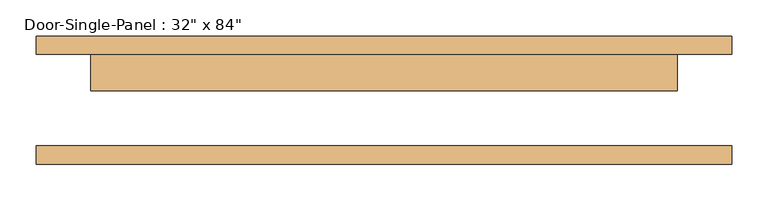
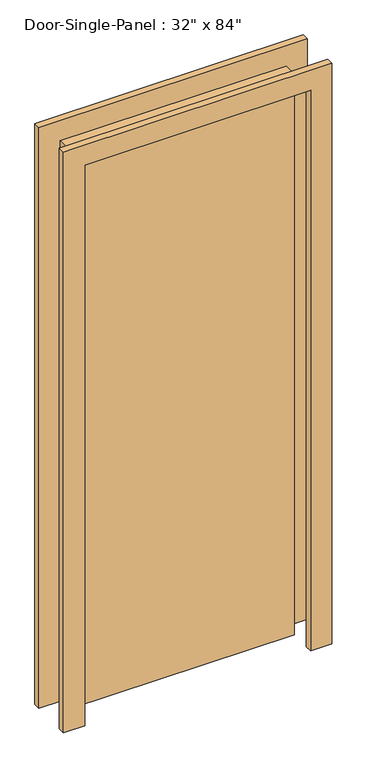
"""IFC4 building model written with IfcOpenShell, lengths in millimetres: door geometry."""

from ifc_helpers import new_model, si_unit, frame, origin, origin_with_axes, place, context, project, spatial, polyline, outline, extrude, source, transform, mapped, element, save


def door_01e03998(model_context):
    return source(origin(), model_context, "Body", "SweptSolid", [
        extrude(outline(polyline([(406.4, 12.7), (-406.4, 12.7), (-406.4, 63.5), (406.4, 63.5), (406.4, 12.7)])), origin_with_axes(), (0.0, 0.0, 1.0), 2133.6),
        extrude(outline(polyline([(2209.8, -482.6), (0.0, -482.6), (0.0, -406.4), (2133.6, -406.4), (2133.6, 406.4), (0.0, 406.4), (0.0, 482.6), (2209.8, 482.6), (2209.8, -482.6)])), frame((0.0, 63.5, 0.0), z_axis=(0.0, 1.0, 0.0), x_axis=(0.0, 0.0, 1.0)), (0.0, 0.0, 1.0), 25.4),
        extrude(outline(polyline([(2209.8, 482.6), (2209.8, -482.6), (0.0, -482.6), (0.0, -406.4), (2133.6, -406.4), (2133.6, 406.4), (0.0, 406.4), (0.0, 482.6), (2209.8, 482.6)])), frame((0.0, -88.9, 0.0), z_axis=(0.0, 1.0, 0.0), x_axis=(0.0, 0.0, 1.0)), (0.0, 0.0, 1.0), 25.4),
    ])


if __name__ == "__main__":
    model = new_model("IFC4")
    model_context = context("Model", 3, world=origin())
    ifc_project = project(units=[si_unit("LENGTHUNIT", "METRE", prefix="MILLI")], contexts=[model_context])
    site = spatial("IfcSite", under=ifc_project)
    building = spatial("IfcBuilding", under=site)
    placement = place(None, origin())
    door_shape = door_01e03998(model_context)
    element("IfcDoor", 1, ObjectType="Door-Single-Panel : 32\" x 84\"", at=placement, inside=building, context=model_context, shape_type="MappedRepresentation", body=[
        mapped(door_shape, transform((0.0, 0.0, 0.0), x_axis=(1.0, 0.0, 0.0), y_axis=(0.0, 1.0, 0.0), z_axis=(0.0, 0.0, 1.0))),
    ])
    save(model, "model.ifc")

# Revit data of these elements
# Type "Door-Single-Panel : 32\" x 84\""
#   Type Mark = "11"
#   Construction Type Id = "DOOR"
#   Assembly Code = "C1020300"
#   Analytic Construction = "Wooden"
#   Thickness = 0' - 2"
#   Thermal Resistance (R) = 2.5876 (h·ft²·°F)/BTU
#   Swing Angle [instance default] = 90.00°
#   Heat Transfer Coefficient (U) = 0.3865 BTU/(h·ft²·°F)
#   Height = 7' - 0"
#   Trim Projection Ext = 0' - 1"
#   Trim Projection Int = 0' - 1"
#   Trim Width = 0' - 3"
#   Width = 2' - 8"
#   Define Thermal Properties by = 1
#   Panel Material = Wood - Birch - Solid Stained Light Low Gloss
#   Trim Material = Paint - Sienna
#   Visual Light Transmittance = 0
#   Solar Heat Gain Coefficient = 0
#   Function = (empty or 0)
#   Wall Closure = (empty or 0)
# Element 1 (IfcDoor, "Door-Single-Panel : 32\" x 84\"")
#   Materials on its faces: "Paint - Sienna", "Wood - Birch - Solid Stained Light Low Gloss"
# Materials
#   "Wood - Birch - Solid Stained Light Low Gloss": class "Wood", colour RGB 210 159 95, transparency 0, Cost = 0
#   "Paint - Sienna": colour RGB 118 70 51, transparency 0, Cost = 0
